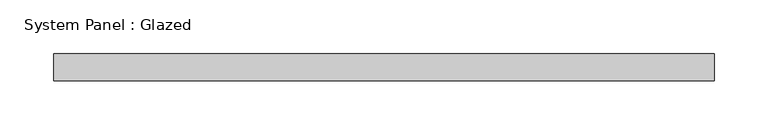
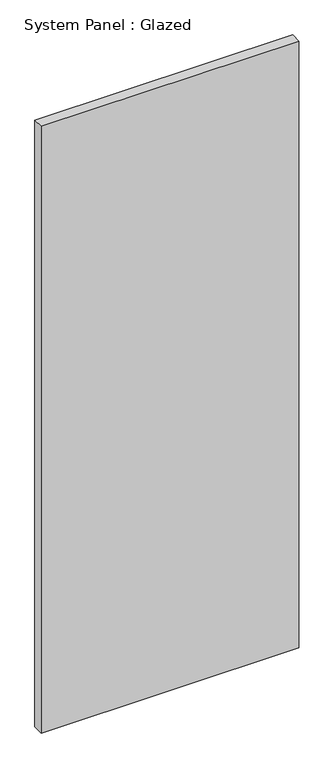
"""IFC4 building model written with IfcOpenShell, lengths in millimetres: plate geometry, System Panel : Glazed."""

from ifc_helpers import new_model, si_unit, origin, origin_with_axes, place, context, project, spatial, polyline, outline, extrude, source, transform, mapped, element, save


def system_panel_glazed_c2bb5d5a(model_context):
    return source(origin(), model_context, "Body", "SweptSolid", [
        extrude(outline(polyline([(307.975, 19.05), (-307.975, 19.05), (-307.975, 44.45), (307.975, 44.45), (307.975, 19.05)])), origin_with_axes(), (0.0, 0.0, 1.0), 1533.012385),
    ])


if __name__ == "__main__":
    model = new_model("IFC4")
    model_context = context("Model", 3, world=origin())
    ifc_project = project(units=[si_unit("LENGTHUNIT", "METRE", prefix="MILLI")], contexts=[model_context])
    site = spatial("IfcSite", under=ifc_project)
    building = spatial("IfcBuilding", under=site)
    placement = place(None, origin())
    system_panel_glazed_shape = system_panel_glazed_c2bb5d5a(model_context)
    element("IfcPlate", 1, ObjectType="System Panel : Glazed", at=placement, inside=building, context=model_context, shape_type="MappedRepresentation", body=[
        mapped(system_panel_glazed_shape, transform((0.0, 0.0, 0.0), x_axis=(1.0, 0.0, 0.0), y_axis=(0.0, 1.0, 0.0), z_axis=(0.0, 0.0, 1.0))),
    ])
    save(model, "model.ifc")

# Revit data of these elements
# Type "System Panel : Glazed"
#   Construction Type Id = "GSP4R"
#   Analytic Construction = "1/8 in Pilkington single glazing"
#   Visual Light Transmittance = 0.9
#   Solar Heat Gain Coefficient = 0.86
#   Heat Transfer Coefficient (U) = 1.18115 BTU/(h·ft²·°F)
#   Define Thermal Properties by = 1
# Element 1 (IfcPlate, "System Panel : Glazed")
#   Materials on its faces: "Glass"
# Materials
#   "Glass": class "Glass", colour RGB 0 128 192, transparency 0.75, Description = "Soda Lime Glass", Cost = 0
